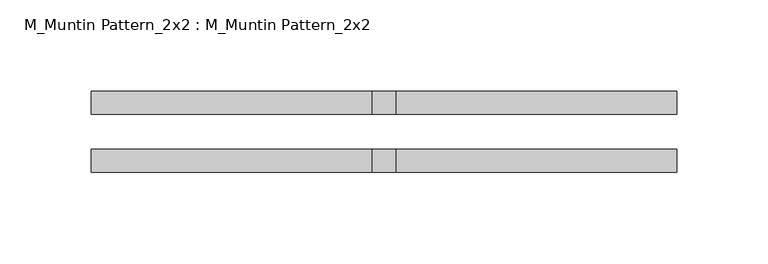
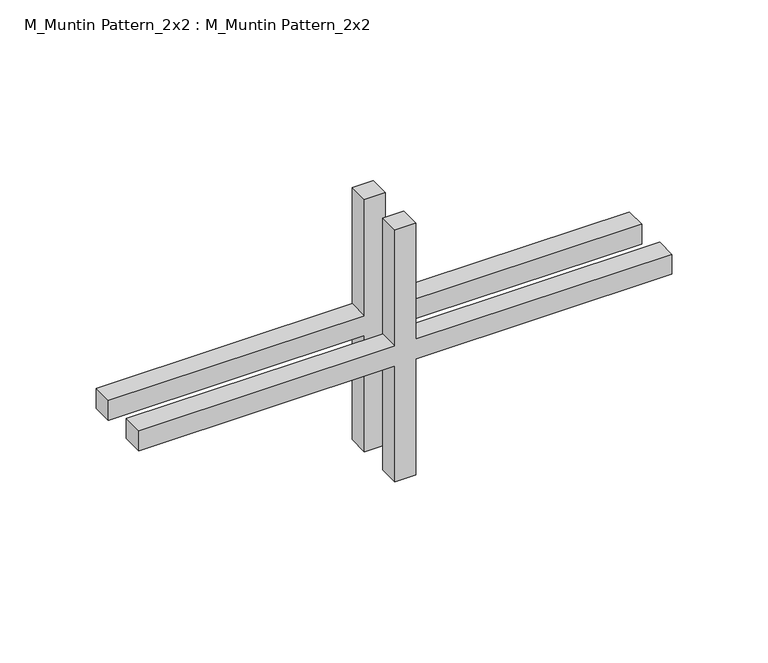
"""IFC4 building model written with IfcOpenShell, lengths in millimetres: proxy geometry, M_Muntin Pattern_2x2 : M_Muntin Pattern_2x2."""

from ifc_helpers import new_model, si_unit, frame, origin, place, context, project, spatial, polyline, outline, extrude, source, transform, mapped, element, save


def m_muntin_pattern_2x2_m_muntin_pattern_2x2_332c70e0(model_context):
    return source(origin(), model_context, "Body", "SweptSolid", [
        extrude(outline(polyline([(86.5, -6.35), (86.5, -160.3375), (73.8, -160.3375), (73.8, -6.35), (0.0, -6.35), (0.0, 6.35), (73.8, 6.35), (73.8, 160.3375), (86.5, 160.3375), (86.5, 6.35), (160.3, 6.35), (160.3, -6.35), (86.5, -6.35)])), frame((0.0, -22.225, 0.0), z_axis=(0.0, 1.0, 0.0), x_axis=(0.0, 0.0, 1.0)), (0.0, 0.0, 1.0), 12.7),
        extrude(outline(polyline([(86.5, -6.35), (86.5, -160.3375), (73.8, -160.3375), (73.8, -6.35), (0.0, -6.35), (0.0, 6.35), (73.8, 6.35), (73.8, 160.3375), (86.5, 160.3375), (86.5, 6.35), (160.3, 6.35), (160.3, -6.35), (86.5, -6.35)])), frame((0.0, 9.525, 0.0), z_axis=(0.0, 1.0, 0.0), x_axis=(0.0, 0.0, 1.0)), (0.0, 0.0, 1.0), 12.7),
    ])


if __name__ == "__main__":
    model = new_model("IFC4")
    model_context = context("Model", 3, world=origin())
    ifc_project = project(units=[si_unit("LENGTHUNIT", "METRE", prefix="MILLI")], contexts=[model_context])
    site = spatial("IfcSite", under=ifc_project)
    building = spatial("IfcBuilding", under=site)
    placement = place(None, origin())
    m_muntin_pattern_2x2_m_muntin_pattern_2x2_shape = m_muntin_pattern_2x2_m_muntin_pattern_2x2_332c70e0(model_context)
    element("IfcBuildingElementProxy", 1, Name="M_Muntin Pattern_2x2 : M_Muntin Pattern_2x2", ObjectType="M_Muntin Pattern_2x2 : M_Muntin Pattern_2x2", at=placement, inside=building, context=model_context, shape_type="MappedRepresentation", body=[
        mapped(m_muntin_pattern_2x2_m_muntin_pattern_2x2_shape, transform((0.0, 0.0, 0.0), x_axis=(1.0, 0.0, 0.0), y_axis=(0.0, 1.0, 0.0), z_axis=(0.0, 0.0, 1.0))),
    ])
    save(model, "model.ifc")

# Revit data of these elements
# Type "M_Muntin Pattern_2x2 : M_Muntin Pattern_2x2"
#   Width [instance default] = 3' - 11.24409"
#   Thickness = 0' - 0 1/2"
#   Height [instance default] = 3' - 11.24409"
#   Distance = 0' - 0 3/4"
#   Interior Material [instance default] = none
#   Exterior Material [instance default] = none
#   Default Elevation = 0
# Element 1 (IfcBuildingElementProxy, "M_Muntin Pattern_2x2 : M_Muntin Pattern_2x2")
#   Width = 1' - 0 5/8"
#   Height = 0' - 6.31102"
#   Interior Material = Wood - Stained
#   Exterior Material = Clad - White
#   Materials on its faces: "Clad - White", "Wood - Stained"
# Materials
#   "Clad - White": class "Wood", colour RGB 242 242 238, transparency 0, Cost = 0
#   "Wood - Stained": class "Wood", colour RGB 224 178 126, transparency 0, Cost = 0
